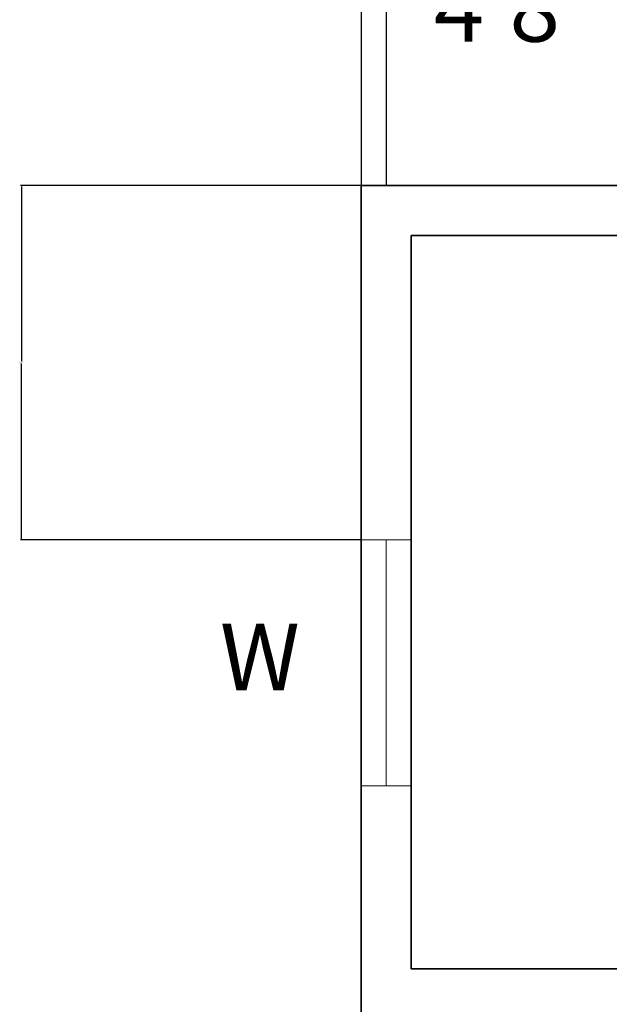
# Model space of a CAD drawing. Units: feet. Extents: x 5816 to 6644, y 25475 to 26788.
# Tile 11 of 23: x 5816 to 5922, y 26514 to 26691. Entities that reach past the tile are written whole.
import ezdxf

# ---------------------------------------------------------------- set-up
doc = ezdxf.new("R2010")
doc.units = ezdxf.units.FT
for name, color, linetype, lineweight in [('A-ANNO-DIMS', 2, 'Continuous', 13), ('A-ANNO-TEXT', 7, 'Continuous', 18), ('A-AREA-IDEN', 7, 'Continuous', 18), ('A-FLOR-RAIL', 8, 'Continuous', 25), ('A-GLAZ', 4, 'Continuous', 18), ('A-WALL', 7, 'Continuous', 35)]:
    doc.layers.add(name, color=color, linetype=linetype, lineweight=lineweight)
doc.styles.get("Standard").update_dxf_attribs({"font": 'arial.ttf'})
doc.dimstyles.get("Standard").update_dxf_attribs({"dimtxt": 0.18, "dimasz": 0.18, "dimexe": 0.18, "dimexo": 0.0625, "dimgap": 0.09, "dimtad": 0, "dimtih": 1, "dimtoh": 1, "dimdec": 4, "dimzin": 0, "dimdsep": 46, "dimtxsty": 'Standard', "dimcen": 0.09, "dimadec": 0, "dimazin": 0, "dimtfac": 1, "dimtdec": 4, "dimtofl": 0, "dimtmove": 0, "dimatfit": 3, "dimfxl": 1, "dimtolj": 1, "dimtzin": 0, "dimarcsym": 0})

# ---------------------------------------------------------------- blocks, each defined once
blk = doc.blocks.new('WIN-BEDROOM-BALCONY')
for p, q in [((0, 0), (9, 0)), ((4.5, 0), (4.5, -44.28)), ((0, -44.28), (9, -44.28))]:
    blk.add_line(p, q)
blk = doc.blocks.new('RAIL-BALCONY-CORNER')
for p, q in [((0, 0), (0, -65)), ((0, 0), (195, 0)), ((4.5, -4.5), (4.5, -65)), ((4.5, -4.5), (195, -4.5))]:
    blk.add_line(p, q)
blk = doc.blocks.new('*D64')
at = {"layer": 'A-ANNO-DIMS', "color": 0, "lineweight": -2, "transparency": 16777216}
for p, q in [((5877.25, 26661.58), (5815.98, 26661.58)), ((5816.16, 26661.4), (5816.16, 26629.87)), ((5816.16, 26597.97), (5816.16, 26629.51)), ((5877.25, 26597.79), (5815.98, 26597.79))]:
    blk.add_line(p, q, dxfattribs=at)
at = {"layer": 'A-ANNO-DIMS', "color": 0, "transparency": 16777216}
for points in [[(5816.13, 26661.4), (5816.19, 26661.4), (5816.16, 26661.58)], [(5816.13, 26597.97), (5816.19, 26597.97), (5816.16, 26597.79)]]:
    blk.add_solid(points, dxfattribs=at)
at = {"layer": 'Defpoints', "color": 0, "transparency": 16777216}
for p in [(5877.31, 26661.58), (5816.16, 26597.79), (5877.31, 26597.79)]:
    blk.add_point(p, dxfattribs=at)
at = {"layer": 'A-ANNO-DIMS', "color": 0, "transparency": 16777216, "insert": (5816.16, 26629.69), "char_height": 0.18, "attachment_point": 5}
blk.add_mtext('\\A1;63.79', dxfattribs=at)

msp = doc.modelspace()

# ---------------------------------------------------------------- linework, layer by layer
at = {"layer": 'A-WALL'}
for p, q in [((5877.3119, 26661.5846), (6048.3119, 26661.5846)), ((5877.3119, 26661.5846), (5877.3119, 26652.5846)), ((5877.3119, 26652.5846), (5877.3119, 26253.5846)), ((5886.3119, 26652.5846), (6048.3119, 26652.5846)), ((5886.3119, 26652.5846), (5886.3119, 26520.5846)), ((5886.3119, 26520.5846), (6081.3119, 26520.5846))]:
    msp.add_line(p, q, dxfattribs=at)

# ---------------------------------------------------------------- block references
at = {"layer": 'A-FLOR-RAIL'}
msp.add_blockref('RAIL-BALCONY-CORNER', (5877.3119, 26726.5846), dxfattribs=at)
at = {"layer": 'A-GLAZ'}
msp.add_blockref('WIN-BEDROOM-BALCONY', (5877.3119, 26597.7938), dxfattribs=at)

# ---------------------------------------------------------------- texts
at = {"layer": 'A-ANNO-TEXT'}
msp.add_text('W', height=12, dxfattribs=at).set_placement((5851.884, 26570.6737))
at = {"layer": 'A-AREA-IDEN'}
msp.add_text('4\'8" WIDE BALCONY', height=12, dxfattribs=at).set_placement((5890.3368, 26687.4804))

# ---------------------------------------------------------------- dimensions: what is measured, and where the dimension line sits
at = {"layer": 'A-ANNO-DIMS'}
dim = msp.add_linear_dim(base=(5816.1619, 26597.7938), p1=(5877.3119, 26661.5846), p2=(5877.3119, 26597.7938), angle=90, dimstyle='Standard', override={"dimdec": 2, "dimlfac": 1, "dimrnd": 0, "dimzin": 0, "dimdsep": 46, "dimlunit": 2}, dxfattribs=at)
dim.commit()
dim.dimension.update_dxf_attribs({"geometry": '*D64', "text_midpoint": (5816.1619, 26629.6892)})

doc.saveas('drawing.dxf')
